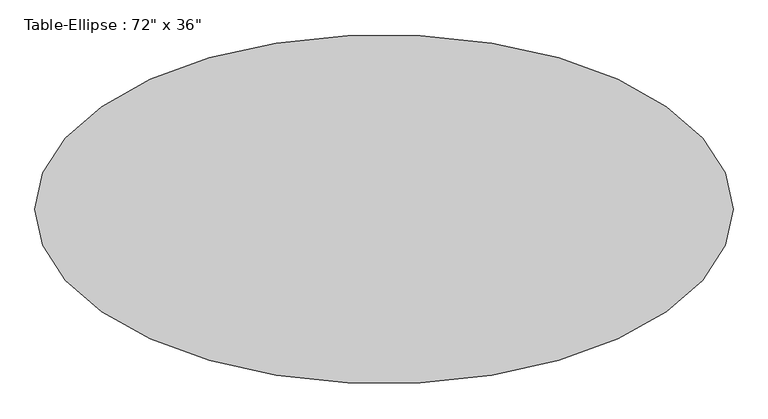
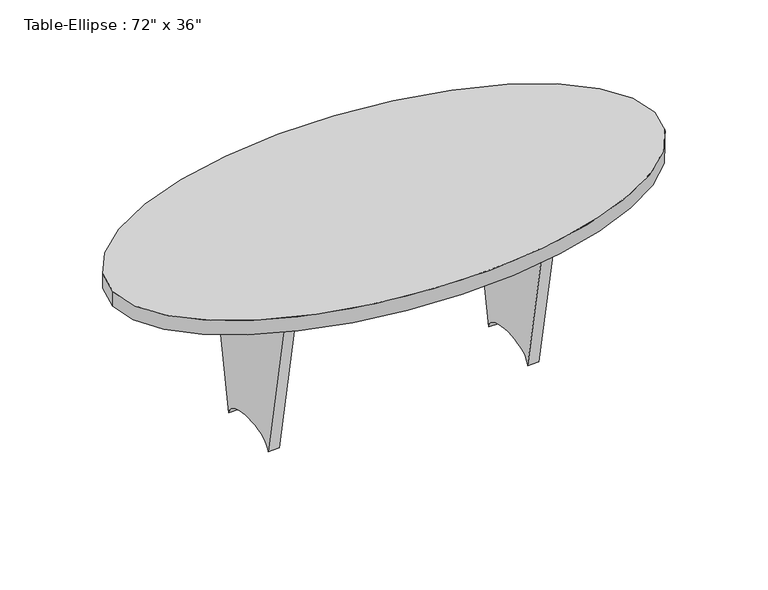
"""IFC4 building model written with IfcOpenShell, lengths in millimetres: furniture geometry."""

from ifc_helpers import new_model, si_unit, point, frame, origin, place, context, project, spatial, ellipse_curve, trimmed, source, transform, mapped, element, save
from ifc_brep_helpers import plane_surface, extruded_surface, advanced_brep


def furniture_962d0db1(model_context):
    return source(origin(), model_context, "Body", "AdvancedBrep", [
        advanced_brep(
        [(-419.1, 19.05, 609.6), (419.1, 19.05, 609.6), (419.1, 19.05, 406.4), (-419.1, 19.05, 406.4), (-419.1, -19.05, 609.6), (-419.1, -19.05, 406.4), (419.1, -19.05, 406.4), (419.1, -19.05, 609.6)],
        [
            (0, 1),
            (1, 2),
            (2, 3, ellipse_curve(frame((0.0, 19.05, 406.4), z_axis=(0.0, -1.0, 0.0), x_axis=(1.0, 0.0, 0.0)), 419.1, 101.6)),
            (3, 0),
            (4, 5),
            (5, 6, ellipse_curve(frame((0.0, -19.05, 406.4), z_axis=(0.0, 1.0, 0.0), x_axis=(1.0, 0.0, 0.0)), 419.1, 101.6)),
            (6, 7),
            (7, 4),
            (0, 4),
            (7, 1),
            (6, 2),
            (5, 3),
        ],
        [
            plane_surface(frame((-419.1, 19.05, 609.6), z_axis=(0.0, 1.0, 0.0), x_axis=(1.0, 0.0, 0.0))),
            plane_surface(frame((-419.1, -19.05, 609.6), z_axis=(0.0, -1.0, 0.0), x_axis=(-1.0, 0.0, 0.0))),
            plane_surface(frame((-419.1, 19.05, 609.6), z_axis=(0.0, 0.0, 1.0), x_axis=(0.0, -1.0, 0.0))),
            plane_surface(frame((419.1, 19.05, 609.6), z_axis=(1.0, 0.0, 0.0), x_axis=(0.0, -1.0, 0.0))),
            extruded_surface(trimmed(ellipse_curve(frame((0.0, -57.15, 406.4), z_axis=(0.0, -1.0, 0.0), x_axis=(1.0, 0.0, 0.0)), 419.1, 101.6), [point((419.1, -57.15, 406.4))], [point((-419.1, -57.15, 406.4))], True, "CARTESIAN"), (0.0, 38.099999999999994, 0.0), 38.099999999999994),
            plane_surface(frame((-419.1, 19.05, 406.4), z_axis=(-1.0, 0.0, 0.0), x_axis=(0.0, -1.0, 0.0))),
        ],
        [
            (0, [[1, 2, 3, 4]]),
            (1, [[5, 6, 7, 8]]),
            (2, [[-1, 9, -8, 10]]),
            (3, [[-2, -10, -7, 11]]),
            (4, [[-3, -11, -6, 12]]),
            (5, [[-4, -12, -5, -9]]),
        ],
    ),
        advanced_brep(
        [(457.2, 228.6, 609.6), (457.2, -228.6, 609.6), (457.2, -114.3, 0.0), (457.2, 114.3, 0.0), (419.1, 228.6, 609.6), (419.1, 114.3, 0.0), (419.1, -114.3, 0.0), (419.1, -228.6, 609.6)],
        [
            (0, 1),
            (1, 2),
            (2, 3, ellipse_curve(frame((457.2, 0.0, 0.0), z_axis=(-1.0, 0.0, 0.0), x_axis=(0.0, 1.0, 0.0)), 114.3, 50.8)),
            (3, 0),
            (4, 5),
            (5, 6, ellipse_curve(frame((419.1, 0.0, 0.0), z_axis=(1.0, 0.0, 0.0), x_axis=(0.0, 1.0, 0.0)), 114.3, 50.8)),
            (6, 7),
            (7, 4),
            (0, 4),
            (7, 1),
            (6, 2),
            (5, 3),
        ],
        [
            plane_surface(frame((457.2, -228.6, 609.6), z_axis=(1.0, 0.0, 0.0), x_axis=(0.0, -1.0, 0.0))),
            plane_surface(frame((419.1, -228.6, 609.6), z_axis=(-1.0, 0.0, 0.0), x_axis=(0.0, 1.0, 0.0))),
            plane_surface(frame((457.2, 228.6, 609.6), z_axis=(0.0, 0.0, 1.0), x_axis=(-1.0, 0.0, 0.0))),
            plane_surface(frame((457.2, -228.6, 609.6), z_axis=(0.0, -0.9828721869343205, -0.18428853505019288), x_axis=(-1.0, 0.0, 0.0))),
            extruded_surface(trimmed(ellipse_curve(frame((381.0, 0.0, 0.0), z_axis=(-1.0, 0.0, 0.0), x_axis=(0.0, 1.0, 0.0)), 114.3, 50.8), [point((381.0, -114.3, 0.0))], [point((381.0, 114.3, 0.0))], True, "CARTESIAN"), (38.10000000000002, 0.0, 0.0), 38.10000000000002),
            plane_surface(frame((457.2, 114.3, 0.0), z_axis=(0.0, 0.9828721869343239, -0.18428853505017528), x_axis=(-1.0, 0.0, 0.0))),
        ],
        [
            (0, [[1, 2, 3, 4]]),
            (1, [[5, 6, 7, 8]]),
            (2, [[-1, 9, -8, 10]]),
            (3, [[-2, -10, -7, 11]]),
            (4, [[-3, -11, -6, 12]]),
            (5, [[-4, -12, -5, -9]]),
        ],
    ),
        advanced_brep(
        [(-419.1, 228.6, 609.6), (-419.1, -228.6, 609.6), (-419.1, -114.3, 0.0), (-419.1, 114.3, 0.0), (-457.2, 228.6, 609.6), (-457.2, 114.3, 0.0), (-457.2, -114.3, 0.0), (-457.2, -228.6, 609.6)],
        [
            (0, 1),
            (1, 2),
            (2, 3, ellipse_curve(frame((-419.1, 0.0, 0.0), z_axis=(-1.0, 0.0, 0.0), x_axis=(0.0, 1.0, 0.0)), 114.3, 50.8)),
            (3, 0),
            (4, 5),
            (5, 6, ellipse_curve(frame((-457.2, 0.0, 0.0), z_axis=(1.0, 0.0, 0.0), x_axis=(0.0, 1.0, 0.0)), 114.3, 50.8)),
            (6, 7),
            (7, 4),
            (0, 4),
            (7, 1),
            (6, 2),
            (5, 3),
        ],
        [
            plane_surface(frame((-419.1, -228.6, 609.6), z_axis=(1.0, 0.0, 0.0), x_axis=(0.0, -1.0, 0.0))),
            plane_surface(frame((-457.2, -228.6, 609.6), z_axis=(-1.0, 0.0, 0.0), x_axis=(0.0, 1.0, 0.0))),
            plane_surface(frame((-419.1, 228.6, 609.6), z_axis=(0.0, 0.0, 1.0), x_axis=(-1.0, 0.0, 0.0))),
            plane_surface(frame((-419.1, -228.6, 609.6), z_axis=(0.0, -0.9828721869343208, -0.18428853505019174), x_axis=(-1.0, 0.0, 0.0))),
            extruded_surface(trimmed(ellipse_curve(frame((-495.3, 0.0, 0.0), z_axis=(-1.0, 0.0, 0.0), x_axis=(0.0, 1.0, 0.0)), 114.3, 50.8), [point((-495.3, -114.3, 0.0))], [point((-495.3, 114.3, 0.0))], True, "CARTESIAN"), (38.10000000000002, 0.0, 0.0), 38.10000000000002),
            plane_surface(frame((-419.1, 114.3, 0.0), z_axis=(0.0, 0.9828721869343228, -0.18428853505018128), x_axis=(-1.0, 0.0, 0.0))),
        ],
        [
            (0, [[1, 2, 3, 4]]),
            (1, [[5, 6, 7, 8]]),
            (2, [[-1, 9, -8, 10]]),
            (3, [[-2, -10, -7, 11]]),
            (4, [[-3, -11, -6, 12]]),
            (5, [[-4, -12, -5, -9]]),
        ],
    ),
        advanced_brep(
        [(-914.4, 0.0, 660.4), (914.4, 0.0, 660.4), (-914.4, 0.0, 609.6), (914.4, 0.0, 609.6)],
        [
            (0, 1, ellipse_curve(frame((0.0, 0.0, 660.4), z_axis=(0.0, 0.0, 1.0), x_axis=(1.0, 0.0, 0.0)), 914.4, 457.2)),
            (1, 0, ellipse_curve(frame((0.0, 0.0, 660.4), z_axis=(0.0, 0.0, 1.0), x_axis=(1.0, 0.0, 0.0)), 914.4, 457.2)),
            (2, 3, ellipse_curve(frame((0.0, 0.0, 609.6), z_axis=(0.0, 0.0, -1.0), x_axis=(1.0, 0.0, 0.0)), 914.4, 457.2)),
            (3, 2, ellipse_curve(frame((0.0, 0.0, 609.6), z_axis=(0.0, 0.0, -1.0), x_axis=(1.0, 0.0, 0.0)), 914.4, 457.2)),
            (0, 2),
            (3, 1),
        ],
        [
            plane_surface(frame((914.4, 0.0, 660.4), z_axis=(0.0, 0.0, 1.0), x_axis=(0.0, 1.0, 0.0))),
            plane_surface(frame((914.4, 0.0, 609.6), z_axis=(0.0, 0.0, -1.0), x_axis=(0.0, -1.0, 0.0))),
            extruded_surface(trimmed(ellipse_curve(frame((0.0, 0.0, 558.8), z_axis=(0.0, 0.0, 1.0), x_axis=(1.0, 0.0, 0.0)), 914.4, 457.2), [point((-914.4, 0.0, 558.8))], [point((914.4, 0.0, 558.8))], True, "CARTESIAN"), (0.0, 0.0, 50.80000000000007), 50.80000000000007),
            extruded_surface(trimmed(ellipse_curve(frame((0.0, 0.0, 558.8), z_axis=(0.0, 0.0, 1.0), x_axis=(1.0, 0.0, 0.0)), 914.4, 457.2), [point((914.4, 0.0, 558.8))], [point((-914.4, 0.0, 558.8))], True, "CARTESIAN"), (0.0, 0.0, 50.80000000000007), 50.80000000000007),
        ],
        [
            (0, [[1, 2]]),
            (1, [[3, 4]]),
            (2, [[-1, 5, -4, 6]]),
            (3, [[-2, -6, -3, -5]]),
        ],
    ),
    ])


if __name__ == "__main__":
    model = new_model("IFC4")
    model_context = context("Model", 3, world=origin())
    ifc_project = project(units=[si_unit("LENGTHUNIT", "METRE", prefix="MILLI")], contexts=[model_context])
    site = spatial("IfcSite", under=ifc_project)
    building = spatial("IfcBuilding", under=site)
    placement = place(None, origin())
    furniture_shape = furniture_962d0db1(model_context)
    element("IfcFurniture", 1, ObjectType="Table-Ellipse : 72\" x 36\"", at=placement, inside=building, context=model_context, shape_type="MappedRepresentation", body=[
        mapped(furniture_shape, transform((0.0, 0.0, 0.0), x_axis=(1.0, 0.0, 0.0), y_axis=(0.0, 1.0, 0.0), z_axis=(0.0, 0.0, 1.0))),
    ])
    save(model, "model.ifc")

# Revit data of these elements
# Type "Table-Ellipse : 72\" x 36\""
#   Assembly Code = "E2020200"
#   Half Width = 1' - 6"
#   Half Length = 3' - 0"
#   Height = 2' - 2"
#   Length = 6' - 0"
#   Width = 3' - 0"
#   Base Material = Birch
#   Top Material = Plywood, Sheathing
#   Default Elevation = 0
# Element 1 (IfcFurniture, "Table-Ellipse : 72\" x 36\"")
#   Materials on its faces: "Birch", "Plywood, Sheathing"
# Materials
#   "Birch": class "Wood", colour RGB 210 159 95, transparency 0, Description = "Betula Alleghaniensis", Cost = 0
#   "Plywood, Sheathing": class "Wood", colour RGB 212 179 113, transparency 0, Description = "Plywood, sheathing grade", Cost = 0
